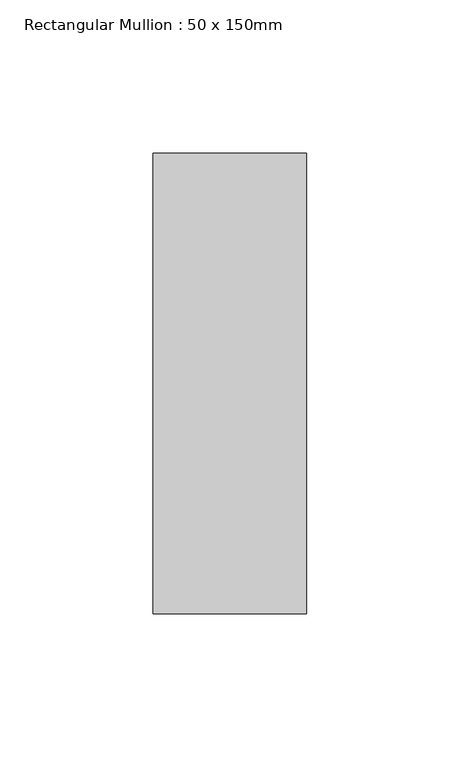
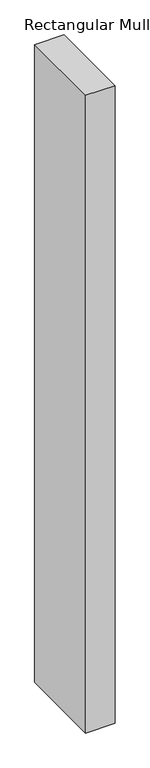
"""IFC4 building model written with IfcOpenShell, lengths in millimetres: member geometry, Rectangular Mullion : 50 x 150mm."""

from ifc_helpers import new_model, si_unit, frame, origin, place, context, project, spatial, polyline, outline, extrude, source, transform, mapped, element, save


def rectangular_mullion_50_x_150mm_7b2d4eb8(model_context):
    return source(origin(), model_context, "Body", "SweptSolid", [
        extrude(outline(polyline([(0.0, 75.0), (0.0, -75.0), (-50.0, -75.0), (-50.0, 75.0), (0.0, 75.0)])), frame((0.0, 0.0, -1144.2), z_axis=(0.0, 0.0, 1.0), x_axis=(1.0, 0.0, 0.0)), (0.0, 0.0, 1.0), 1144.2),
    ])


if __name__ == "__main__":
    model = new_model("IFC4")
    model_context = context("Model", 3, world=origin())
    ifc_project = project(units=[si_unit("LENGTHUNIT", "METRE", prefix="MILLI")], contexts=[model_context])
    site = spatial("IfcSite", under=ifc_project)
    building = spatial("IfcBuilding", under=site)
    placement = place(None, origin())
    rectangular_mullion_50_x_150mm_shape = rectangular_mullion_50_x_150mm_7b2d4eb8(model_context)
    element("IfcMember", 1, ObjectType="Rectangular Mullion : 50 x 150mm", at=placement, inside=building, context=model_context, shape_type="MappedRepresentation", body=[
        mapped(rectangular_mullion_50_x_150mm_shape, transform((0.0, 0.0, 0.0), x_axis=(1.0, 0.0, 0.0), y_axis=(0.0, 1.0, 0.0), z_axis=(0.0, 0.0, 1.0))),
    ])
    save(model, "model.ifc")

# Revit data of these elements
# Type "Rectangular Mullion : 50 x 150mm"
#   built-in parameter 1007304 = 0.492126 (stored number, unit not read)
#   built-in parameter 1007301 = 0.082021 (stored number, unit not read)
#   built-in parameter 1007300 = 0.082021 (stored number, unit not read)
# Element 1 (IfcMember, "Rectangular Mullion : 50 x 150mm")
#   Materials on its faces: "Aluminium"
# Materials
#   "Aluminium": class "Metal", colour RGB 247 247 247, transparency 0, Description = "Aluminium 6061", Cost = 0
